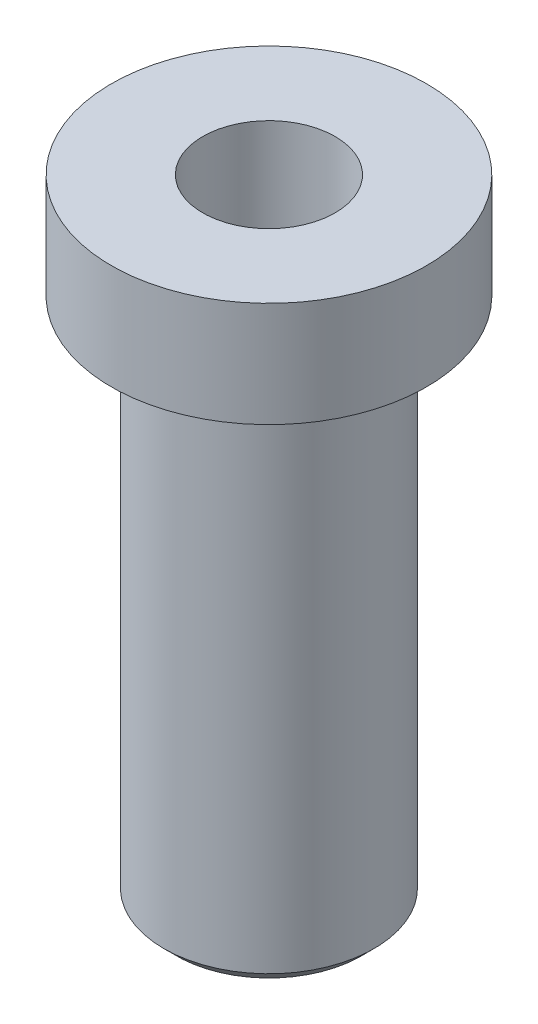
ISO-10303-21;
HEADER;
FILE_DESCRIPTION(('STEP AP214'),'2;1');
FILE_NAME('part.step','',(''),(''),'','','');
FILE_SCHEMA(('AUTOMOTIVE_DESIGN { 1 0 10303 214 1 1 1 1 }'));
ENDSEC;
DATA;
#1=APPLICATION_CONTEXT('core data for automotive mechanical design processes');
#2=APPLICATION_PROTOCOL_DEFINITION('international standard','automotive_design',2000,#1);
#3=PRODUCT_CONTEXT('',#1,'mechanical');
#4=PRODUCT('Part','Part','',(#3));
#5=PRODUCT_RELATED_PRODUCT_CATEGORY('part','',(#4));
#6=PRODUCT_DEFINITION_FORMATION('','',#4);
#7=PRODUCT_DEFINITION_CONTEXT('part definition',#1,'design');
#8=PRODUCT_DEFINITION('design','',#6,#7);
#9=PRODUCT_DEFINITION_SHAPE('','',#8);
#10=(LENGTH_UNIT() NAMED_UNIT(*) SI_UNIT(.MILLI.,.METRE.));
#11=(NAMED_UNIT(*) PLANE_ANGLE_UNIT() SI_UNIT($,.RADIAN.));
#12=(NAMED_UNIT(*) SI_UNIT($,.STERADIAN.) SOLID_ANGLE_UNIT());
#13=UNCERTAINTY_MEASURE_WITH_UNIT(LENGTH_MEASURE(1.E-05),#10,'distance_accuracy_value','');
#14=(GEOMETRIC_REPRESENTATION_CONTEXT(3) GLOBAL_UNCERTAINTY_ASSIGNED_CONTEXT((#13)) GLOBAL_UNIT_ASSIGNED_CONTEXT((#10,
#11,#12)) REPRESENTATION_CONTEXT('',''));
#15=CARTESIAN_POINT('',(0.,0.,0.));
#16=DIRECTION('',(0.,0.,1.));
#17=DIRECTION('',(1.,0.,0.));
#18=AXIS2_PLACEMENT_3D('',#15,#16,#17);
#19=CARTESIAN_POINT('',(50.,0.,0.));
#20=DIRECTION('',(0.,-1.,0.));
#21=DIRECTION('',(0.,0.,-1.));
#22=AXIS2_PLACEMENT_3D('',#19,#20,#21);
#23=PLANE('',#22);
#24=CARTESIAN_POINT('',(0.,0.,0.));
#25=DIRECTION('',(0.,-1.,0.));
#26=DIRECTION('',(0.,0.,-1.));
#27=AXIS2_PLACEMENT_3D('',#24,#25,#26);
#28=CIRCLE('',#27,44.0000000000001);
#29=CARTESIAN_POINT('',(0.,0.,-44.0000000000001));
#30=VERTEX_POINT('',#29);
#31=EDGE_CURVE('E50',#30,#30,#28,.T.);
#32=ORIENTED_EDGE('',*,*,#31,.T.);
#33=EDGE_LOOP('',(#32));
#34=FACE_BOUND('',#33,.T.);
#35=CARTESIAN_POINT('',(0.,0.,0.));
#36=DIRECTION('',(0.,-1.,0.));
#37=DIRECTION('',(0.,0.,-1.));
#38=AXIS2_PLACEMENT_3D('',#35,#36,#37);
#39=CIRCLE('',#38,31.5);
#40=CARTESIAN_POINT('',(0.,0.,-31.5));
#41=VERTEX_POINT('',#40);
#42=EDGE_CURVE('E51',#41,#41,#39,.T.);
#43=ORIENTED_EDGE('',*,*,#42,.F.);
#44=EDGE_LOOP('',(#43));
#45=FACE_BOUND('',#44,.T.);
#46=ADVANCED_FACE('F39',(#34,#45),#23,.T.);
#47=CARTESIAN_POINT('',(0.,0.,0.));
#48=DIRECTION('',(0.,-1.,0.));
#49=DIRECTION('',(0.,0.,-1.));
#50=AXIS2_PLACEMENT_3D('',#47,#48,#49);
#51=CYLINDRICAL_SURFACE('',#50,31.5);
#52=ORIENTED_EDGE('',*,*,#42,.T.);
#53=EDGE_LOOP('',(#52));
#54=FACE_BOUND('',#53,.T.);
#55=CARTESIAN_POINT('',(0.,300.,0.));
#56=DIRECTION('',(0.,-1.,0.));
#57=DIRECTION('',(0.,0.,-1.));
#58=AXIS2_PLACEMENT_3D('',#55,#56,#57);
#59=CIRCLE('',#58,31.5);
#60=CARTESIAN_POINT('',(0.,300.,-31.5));
#61=VERTEX_POINT('',#60);
#62=EDGE_CURVE('E54',#61,#61,#59,.T.);
#63=ORIENTED_EDGE('',*,*,#62,.F.);
#64=EDGE_LOOP('',(#63));
#65=FACE_BOUND('',#64,.T.);
#66=ADVANCED_FACE('F88',(#54,#65),#51,.F.);
#67=CARTESIAN_POINT('',(31.5,300.,0.));
#68=DIRECTION('',(0.,1.,0.));
#69=DIRECTION('',(0.,0.,1.));
#70=AXIS2_PLACEMENT_3D('',#67,#68,#69);
#71=PLANE('',#70);
#72=ORIENTED_EDGE('',*,*,#62,.T.);
#73=EDGE_LOOP('',(#72));
#74=FACE_BOUND('',#73,.T.);
#75=CARTESIAN_POINT('',(0.,300.,0.));
#76=DIRECTION('',(0.,-1.,0.));
#77=DIRECTION('',(0.,0.,-1.));
#78=AXIS2_PLACEMENT_3D('',#75,#76,#77);
#79=CIRCLE('',#78,75.);
#80=CARTESIAN_POINT('',(0.,300.,-75.));
#81=VERTEX_POINT('',#80);
#82=EDGE_CURVE('E58',#81,#81,#79,.T.);
#83=ORIENTED_EDGE('',*,*,#82,.F.);
#84=EDGE_LOOP('',(#83));
#85=FACE_BOUND('',#84,.T.);
#86=ADVANCED_FACE('F83',(#74,#85),#71,.T.);
#87=CARTESIAN_POINT('',(0.,0.,0.));
#88=DIRECTION('',(0.,-1.,0.));
#89=DIRECTION('',(0.,0.,-1.));
#90=AXIS2_PLACEMENT_3D('',#87,#88,#89);
#91=CYLINDRICAL_SURFACE('',#90,75.);
#92=ORIENTED_EDGE('',*,*,#82,.T.);
#93=EDGE_LOOP('',(#92));
#94=FACE_BOUND('',#93,.T.);
#95=CARTESIAN_POINT('',(0.,250.,0.));
#96=DIRECTION('',(0.,-1.,0.));
#97=DIRECTION('',(0.,0.,-1.));
#98=AXIS2_PLACEMENT_3D('',#95,#96,#97);
#99=CIRCLE('',#98,75.);
#100=CARTESIAN_POINT('',(0.,250.,-75.));
#101=VERTEX_POINT('',#100);
#102=EDGE_CURVE('E64',#101,#101,#99,.T.);
#103=ORIENTED_EDGE('',*,*,#102,.F.);
#104=EDGE_LOOP('',(#103));
#105=FACE_BOUND('',#104,.T.);
#106=ADVANCED_FACE('F74',(#94,#105),#91,.T.);
#107=CARTESIAN_POINT('',(50.,250.,0.));
#108=DIRECTION('',(0.,-1.,0.));
#109=DIRECTION('',(0.,0.,-1.));
#110=AXIS2_PLACEMENT_3D('',#107,#108,#109);
#111=PLANE('',#110);
#112=ORIENTED_EDGE('',*,*,#102,.T.);
#113=EDGE_LOOP('',(#112));
#114=FACE_BOUND('',#113,.T.);
#115=CARTESIAN_POINT('',(0.,250.,0.));
#116=DIRECTION('',(0.,-1.,0.));
#117=DIRECTION('',(0.,0.,-1.));
#118=AXIS2_PLACEMENT_3D('',#115,#116,#117);
#119=CIRCLE('',#118,50.);
#120=CARTESIAN_POINT('',(0.,250.,-50.));
#121=VERTEX_POINT('',#120);
#122=EDGE_CURVE('E67',#121,#121,#119,.T.);
#123=ORIENTED_EDGE('',*,*,#122,.F.);
#124=EDGE_LOOP('',(#123));
#125=FACE_BOUND('',#124,.T.);
#126=ADVANCED_FACE('F75',(#114,#125),#111,.T.);
#127=CARTESIAN_POINT('',(0.,0.,0.));
#128=DIRECTION('',(0.,-1.,0.));
#129=DIRECTION('',(0.,0.,-1.));
#130=AXIS2_PLACEMENT_3D('',#127,#128,#129);
#131=CYLINDRICAL_SURFACE('',#130,50.);
#132=CARTESIAN_POINT('',(0.,5.99999999999996,0.));
#133=DIRECTION('',(0.,-1.,0.));
#134=DIRECTION('',(0.,0.,-1.));
#135=AXIS2_PLACEMENT_3D('',#132,#133,#134);
#136=CIRCLE('',#135,50.);
#137=CARTESIAN_POINT('',(0.,5.99999999999996,-50.));
#138=VERTEX_POINT('',#137);
#139=EDGE_CURVE('E10',#138,#138,#136,.F.);
#140=ORIENTED_EDGE('',*,*,#139,.T.);
#141=EDGE_LOOP('',(#140));
#142=FACE_BOUND('',#141,.T.);
#143=ORIENTED_EDGE('',*,*,#122,.T.);
#144=EDGE_LOOP('',(#143));
#145=FACE_BOUND('',#144,.T.);
#146=ADVANCED_FACE('F66',(#142,#145),#131,.T.);
#147=CARTESIAN_POINT('',(0.,0.,0.));
#148=DIRECTION('',(0.,1.,0.));
#149=DIRECTION('',(0.,0.,1.));
#150=AXIS2_PLACEMENT_3D('',#147,#148,#149);
#151=CONICAL_SURFACE('',#150,44.0000000000001,0.785398163397448);
#152=ORIENTED_EDGE('',*,*,#139,.F.);
#153=EDGE_LOOP('',(#152));
#154=FACE_BOUND('',#153,.T.);
#155=ORIENTED_EDGE('',*,*,#31,.F.);
#156=EDGE_LOOP('',(#155));
#157=FACE_BOUND('',#156,.T.);
#158=ADVANCED_FACE('F45',(#154,#157),#151,.T.);
#159=CLOSED_SHELL('',(#46,#66,#86,#106,#126,#146,#158));
#160=MANIFOLD_SOLID_BREP('B2',#159);
#161=ADVANCED_BREP_SHAPE_REPRESENTATION('',(#18,#160),#14);
#162=SHAPE_DEFINITION_REPRESENTATION(#9,#161);
ENDSEC;
END-ISO-10303-21;
